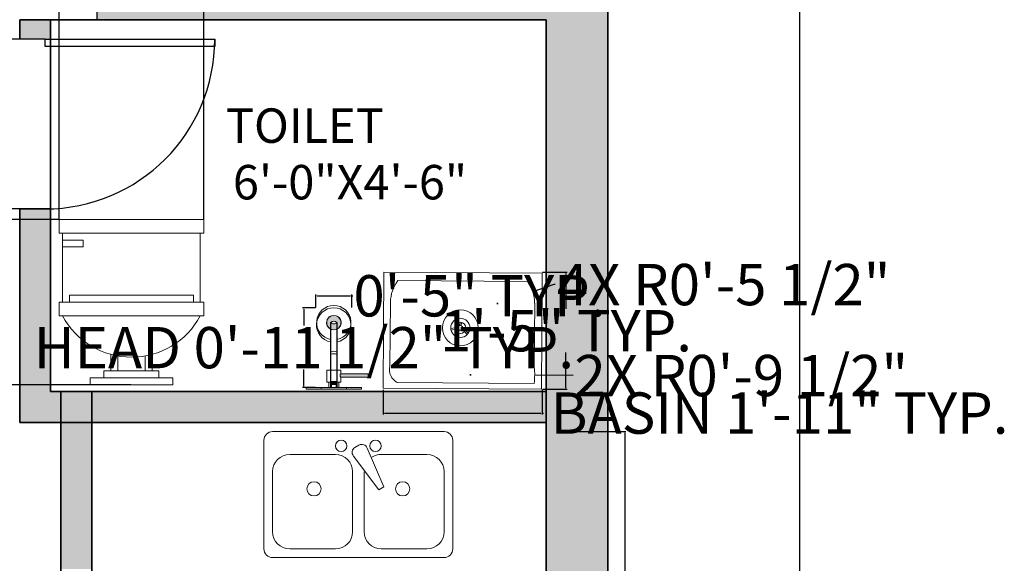
# Model space of a CAD drawing. Units: inches. Extents: x 143233372 to 143233714, y 112671713 to 112672292.
# Tile 5 of 7: x 143233571 to 143233714, y 112672013 to 112672092. Entities that reach past the tile are written whole.
import ezdxf

# ---------------------------------------------------------------- set-up
doc = ezdxf.new("R2010")
doc.units = ezdxf.units.IN
doc.header["$MEASUREMENT"] = 0
doc.layers.get('0').update_dxf_attribs({"color": 104})
for name, color, linetype, lineweight in [('A-ANNO-DIMS', 2, 'Continuous', 18), ('A-AREA-IDEN', 7, 'Continuous', 18), ('doors', 32, 'Continuous', 25), ('PLUMBING FIXTURES', 8, 'Continuous', 18), ('walls', 7, 'Continuous', 35)]:
    doc.layers.add(name, color=color, linetype=linetype, lineweight=lineweight)
doc.layers.add('A-WALL-PATT', color=18, linetype='Continuous', lineweight=9, true_color=0x000000)
doc.styles.add('ATT', font='TXT')
doc.styles.get("Standard").update_dxf_attribs({"font": 'arial.ttf'})
doc.dimstyles.get("Standard").update_dxf_attribs({"dimtxt": 6, "dimasz": 0.18, "dimexe": 0.18, "dimexo": 0.0625, "dimgap": 0.09, "dimtad": 0, "dimtih": 1, "dimtoh": 1, "dimzin": 0, "dimdsep": 46, "dimlunit": 3, "dimtxsty": 'Standard', "dimcen": 0.09, "dimadec": 0, "dimazin": 0, "dimtfac": 1, "dimtofl": 0, "dimtmove": 0, "dimatfit": 3, "dimfxl": 1, "dimtolj": 1, "dimtzin": 0, "dimarcsym": 0})

# ---------------------------------------------------------------- blocks, each defined once
blk = doc.blocks.new('15PSNK10')
at = {"color": 0, "linetype": 'ByBlock'}
for p, q in [((20.5, 16.5), (1.5, 16.5)), ((0, 15), (0, -15)), ((7, 15), (17.5, 15)), ((22, -15), (22, 15)), ((4, 4), (4, 12)), ((20.5, 12), (20.5, 4)), ((2.37, -0.1), (2.77, 0.6)), ((10.18, -3.57), (4.27, 0.87)), ((17.5, 1), (7, 1)), ((2.88, -1.54), (9.68, -4.43)), ((7.04, -1), (17.5, -1)), ((4, -12), (4, -4)), ((9.68, -4.43), (10.18, -3.57)), ((20.5, -4), (20.5, -12)), ((17.5, -15), (7, -15)), ((1.5, -16.5), (20.5, -16.5))]:
    blk.add_line(p, q, dxfattribs=at)
for centre, radius in [((10, 7.75), 1.25), ((2.5, 3), 1), ((2.5, -3), 1), ((10, -7.75), 1.25)]:
    blk.add_circle(centre, radius, dxfattribs=at)
for centre, radius, start, end in [((1.5, 15), 1.5, 90, 180), ((20.5, 15), 1.5, 0, 90), ((7, 12), 3, 90, 180), ((17.5, 12), 3, 0, 90), ((7, 4), 3, 180, 270), ((17.5, 4), 3, 270, 0), ((3.63, 0.1), 1, 50.5377, 150), ((3.23, -0.6), 1, 150, 249.4623), ((17.5, -4), 3, 0, 90), ((7, -4), 3, 146.607, 180), ((7, -12), 3, 180, 270), ((17.5, -12), 3, 270, 0), ((1.5, -15), 1.5, 180, 270), ((20.5, -15), 1.5, 270, 0)]:
    blk.add_arc(centre, radius, start, end, dxfattribs=at)
at = {"color": 0, "linetype": 'ByBlock', "style": 'ATT'}
for tag, p, flags in [('ITEM', (0, -26), 3), ('ROOM_NUMBER', (0, -35), 1)]:
    blk.add_attdef(tag, p, '', height=6, dxfattribs=dict(at, flags=flags))
blk = doc.blocks.new('*U19')
for p, q in [((-10, 22), (-10, 12)), ((10, 12), (10, 22)), ((-10, 21), (-7, 21)), ((-7, 21), (-7, 20)), ((-7, 20), (-10, 20)), ((9, 13), (-9, 13)), ((-9, 13), (-9, 12)), ((9, 12), (9, 13)), ((10.5, 12), (-10.5, 12)), ((-10.5, 10), (-10.5, 12)), ((10.5, 12), (10.5, 10)), ((10.5, 10), (-10.5, 10)), ((-3, 4.4065), (-3, 2)), ((3, 2), (3, 4.4065)), ((-2, 2), (-2, 4.1658)), ((2, 4.1658), (2, 2)), ((4, 2), (-4, 2)), ((-4, 2), (-4, 1)), ((4, 1), (4, 2))]:
    blk.add_line(p, q)
for points in [[(10.5, 22), (10.5, 24), (-10.5, 24), (-10.5, 22)], [(6, 0), (6, 1), (-6, 1), (-6, 0)]]:
    blk.add_lwpolyline(points, close=True)
blk.add_arc((0, 15.3333), 11.3333, 208.0725, 331.9275)
blk = doc.blocks.new('O.H SHOWER-PL')
at = {"layer": 'PLUMBING FIXTURES'}
for points in [[(-1.84, 0), (-1.84, -0.25), (1.84, -0.25), (1.84, 0)], [(0.46, -8.72), (0.46, -9.67, -0.422337), (-0.46, -9.67), (-0.46, -8.72, 4.325472)]]:
    blk.add_hatch(color=256, dxfattribs=at).paths.add_polyline_path(points)
for p, q in [((-1.84, 0), (-1.84, -0.25)), ((1.84, 0), (-1.84, 0)), ((1.84, 0), (1.84, -0.25)), ((1.84, -0.25), (-1.84, -0.25)), ((-0.46, -0.25), (-0.46, -9.67)), ((0.46, -0.25), (0.46, -9.67))]:
    blk.add_line(p, q, dxfattribs=at)
for centre, radius, start, end in [((0, -4.48), 1.03, 243.53, 296.47), ((0, -9.67), 2.5, 100.61, 79.39), ((0, -9.67), 1.05, 116.0349, 63.9652), ((0, -9.22), 0.643, 224.2078, 315.7922)]:
    blk.add_arc(centre, radius, start, end, dxfattribs=at)
blk = doc.blocks.new('DIVERTER-PL')
at = {"layer": 'PLUMBING FIXTURES'}
for points in [[(4, 0), (-4, 0), (-4, -0.25), (4, -0.25)], [(0.38, -1.14), (0.38, -0.7), (-0.37, -0.7), (-0.37, -1.14)], [(1, -1.75, 0.30818), (1, -2.25), (5, -2.25), (5, -1.75)]]:
    blk.add_hatch(color=256, dxfattribs=at).paths.add_polyline_path(points)
for p, q in [((-4, 0), (-4, -0.25)), ((-4, 0), (4, 0)), ((4, 0), (4, -0.25)), ((-4, -0.25), (4, -0.25)), ((-4, -0.25), (4, -0.25)), ((-1, -1.05), (-0.37, -1.05)), ((-1, -1.05), (-1, -2.75)), ((-0.75, -0.25), (-0.75, -1.05)), ((-0.37, -0.7), (0.38, -0.7)), ((-0.37, -0.7), (-0.37, -1.14)), ((-0.37, -1.14), (0.38, -1.14)), ((-0.32, -0.7), (-0.32, -0.25)), ((0.32, -0.7), (0.32, -0.25)), ((0.38, -0.7), (0.38, -1.14)), ((0.38, -1.05), (1, -1.05)), ((0.75, -0.25), (0.75, -1.05)), ((1, -1.05), (1, -1.75)), ((-1, -2.75), (1, -2.75)), ((1, -2.25), (1, -2.75))]:
    blk.add_line(p, q, dxfattribs=at)
at = {"layer": 'PLUMBING FIXTURES', "ltscale": 12}
for p, q in [((1, -1.75), (5, -1.75)), ((1, -2.25), (5, -2.25)), ((5, -2.25), (5, -1.75))]:
    blk.add_line(p, q, dxfattribs=at)
at = {"layer": 'PLUMBING FIXTURES'}
blk.add_arc((1.37, -2), 0.444, 145.7435, 214.2565, dxfattribs=at)
blk = doc.blocks.new('A$C7F153053')
at = {"layer": 'PLUMBING FIXTURES', "xscale": -1, "rotation": 270}
for name in ['DIVERTER-PL', 'O.H SHOWER-PL']:
    blk.add_blockref(name, (12.17, 4), dxfattribs=at)
blk = doc.blocks.new('*U24')
for p, q in [((0, 0), (0, -6)), ((40, 0), (40, -6))]:
    blk.add_line(p, q)
blk.add_lwpolyline([(0, 0), (0, 40), (1.75, 40), (1.75, 0)], close=True)
blk.add_arc((0, 0), 40, 0, 90)
blk = doc.blocks.new('LAVATORY-RECT')
for p, q in [((0, 0.15), (0.11, 17)), ((0.11, 17), (23.11, 16.85)), ((20.97, 15.65), (2.15, 15.77)), ((23.11, 16.85), (23.1, 15.71)), ((23.1, 15.71), (23, 0)), ((0.99, 3.35), (1.05, 12.64)), ((21.96, 3.21), (22.03, 12.5)), ((10.4, 8.91), (9.84, 8.81)), ((10.52, 8.7), (9.87, 8.58)), ((11.22, 9.73), (11.16, 9.24)), ((11.36, 9.22), (11.4, 9.7)), ((11.97, 8.6), (12.36, 8.13)), ((11.84, 8.39), (12.22, 7.95)), ((23, 0), (0, 0.15)), ((21.95, 0.84), (2.06, 0.97))]:
    blk.add_line(p, q)
for radius in [2.61, 1.39, 0.816, 0.338]:
    blk.add_circle((11.22, 8.91), radius)
for centre, radius, start, end in [((6.46, 12.5), 5.4, 142.7525, 178.5493), ((16.62, 12.43), 5.4, 0.6949, 36.4918), ((3, 2.82), 2.08, 165.2338, 242.9258), ((12.7, 2.09), 9.33, 352.3124, 6.9318)]:
    blk.add_arc(centre, radius, start, end)
blk = doc.blocks.new('SHOWER-ARM-AND-HEAD')
blk.add_hatch(color=256).paths.add_polyline_path([(2.05, 10.36), (2.05, 9.42, 0.422337), (2.97, 9.42), (2.97, 10.36, -4.325472)])
blk.add_hatch(color=256).paths.add_polyline_path([(2.05, 10.36), (2.05, 9.42, 0.422337), (2.97, 9.42), (2.97, 10.36, -4.325472)])
blk.add_hatch(color=256).paths.add_polyline_path([(2.05, 10.36), (2.05, 9.42, 0.422337), (2.97, 9.42), (2.97, 10.36, -4.325472)])
blk.add_hatch(color=256).paths.add_polyline_path([(2.05, 10.36), (2.05, 9.42, 0.422337), (2.97, 9.42), (2.97, 10.36, -4.325472)])
blk.add_hatch(color=256).paths.add_polyline_path([(2.05, 10.36), (2.05, 9.42, 0.422337), (2.97, 9.42), (2.97, 10.36, -4.325472)])
blk.add_hatch(color=256).paths.add_polyline_path([(2.05, 10.36), (2.05, 9.42, 0.422337), (2.97, 9.42), (2.97, 10.36, -4.325472)])
blk.add_hatch(color=256).paths.add_polyline_path([(2.05, 10.36), (2.05, 9.42, 0.422337), (2.97, 9.42), (2.97, 10.36, -4.325472)])
blk.add_hatch(color=256).paths.add_polyline_path([(2.05, 10.36), (2.05, 9.42, 0.422337), (2.97, 9.42), (2.97, 10.36, -4.325472)])
blk.add_hatch(color=256).paths.add_polyline_path([(2.05, 10.36), (2.05, 9.42, 0.422337), (2.97, 9.42), (2.97, 10.36, -4.325472)])
blk.add_hatch(color=256).paths.add_polyline_path([(2.05, 10.36), (2.05, 9.42, 0.422337), (2.97, 9.42), (2.97, 10.36, -4.325472)])
blk.add_hatch(color=256).paths.add_polyline_path([(2.05, 10.36), (2.05, 9.42, 0.422337), (2.97, 9.42), (2.97, 10.36, -4.325472)])
blk.add_hatch(color=256).paths.add_polyline_path([(2.05, 10.36), (2.05, 9.42, 0.422337), (2.97, 9.42), (2.97, 10.36, -4.325472)])
blk.add_hatch(color=256).paths.add_polyline_path([(2.05, 10.36), (2.05, 9.42, 0.422337), (2.97, 9.42), (2.97, 10.36, -4.325472)])
blk.add_hatch(color=256).paths.add_polyline_path([(2.05, 10.36), (2.05, 9.42, 0.422337), (2.97, 9.42), (2.97, 10.36, -4.325472)])
blk.add_hatch(color=256).paths.add_polyline_path([(2.05, 10.36), (2.05, 9.42, 0.422337), (2.97, 9.42), (2.97, 10.36, -4.325472)])
blk.add_hatch(color=256).paths.add_polyline_path([(2.05, 10.36), (2.05, 9.42, 0.422337), (2.97, 9.42), (2.97, 10.36, -4.325472)])
blk.add_hatch(color=256).paths.add_polyline_path([(2.05, 10.36), (2.05, 9.42, 0.422337), (2.97, 9.42), (2.97, 10.36, -4.325472)])
blk.add_hatch(color=256).paths.add_polyline_path([(2.05, 10.36), (2.05, 9.42, 0.422337), (2.97, 9.42), (2.97, 10.36, -4.325472)])
blk.add_hatch(color=256).paths.add_polyline_path([(2.05, 10.36), (2.05, 9.42, 0.422337), (2.97, 9.42), (2.97, 10.36, -4.325472)])
blk.add_hatch(color=256).paths.add_polyline_path([(2.05, 10.36), (2.05, 9.42, 0.422337), (2.97, 9.42), (2.97, 10.36, -4.325472)])
blk.add_hatch(color=256).paths.add_polyline_path([(2.05, 10.36), (2.05, 9.42, 0.422337), (2.97, 9.42), (2.97, 10.36, -4.325472)])
blk.add_hatch(color=256).paths.add_polyline_path([(2.05, 10.36), (2.05, 9.42, 0.422337), (2.97, 9.42), (2.97, 10.36, -4.325472)])
blk.add_hatch(color=256).paths.add_polyline_path([(2.05, 10.36), (2.05, 9.42, 0.422337), (2.97, 9.42), (2.97, 10.36, -4.325472)])
blk.add_hatch(color=256).paths.add_polyline_path([(2.05, 10.36), (2.05, 9.42, 0.422337), (2.97, 9.42), (2.97, 10.36, -4.325472)])
blk.add_hatch(color=256).paths.add_polyline_path([(2.05, 10.36), (2.05, 9.42, 0.422337), (2.97, 9.42), (2.97, 10.36, -4.325472)])
blk.add_hatch(color=256).paths.add_polyline_path([(2.05, 10.36), (2.05, 9.42, 0.422337), (2.97, 9.42), (2.97, 10.36, -4.325472)])
blk.add_hatch(color=256).paths.add_polyline_path([(2.05, 10.36), (2.05, 9.42, 0.422337), (2.97, 9.42), (2.97, 10.36, -4.325472)])
blk.add_hatch(color=256).paths.add_polyline_path([(2.05, 10.36), (2.05, 9.42, 0.422337), (2.97, 9.42), (2.97, 10.36, -4.325472)])
blk.add_hatch(color=256).paths.add_polyline_path([(2.05, 10.36), (2.05, 9.42, 0.422337), (2.97, 9.42), (2.97, 10.36, -4.325472)])
blk.add_hatch(color=256).paths.add_polyline_path([(2.05, 10.36), (2.05, 9.42, 0.422337), (2.97, 9.42), (2.97, 10.36, -4.325472)])
blk.add_hatch(color=256).paths.add_polyline_path([(2.05, 10.36), (2.05, 9.42, 0.422337), (2.97, 9.42), (2.97, 10.36, -4.325472)])
blk.add_hatch(color=256).paths.add_polyline_path([(2.05, 10.36), (2.05, 9.42, 0.422337), (2.97, 9.42), (2.97, 10.36, -4.325472)])
blk.add_hatch(color=256).paths.add_polyline_path([(2.05, 10.36), (2.05, 9.42, 0.422337), (2.97, 9.42), (2.97, 10.36, -4.325472)])
blk.add_hatch(color=256).paths.add_polyline_path([(2.05, 10.36), (2.05, 9.42, 0.422337), (2.97, 9.42), (2.97, 10.36, -4.325472)])
blk.add_hatch(color=256).paths.add_polyline_path([(2.05, 10.36), (2.05, 9.42, 0.422337), (2.97, 9.42), (2.97, 10.36, -4.325472)])
blk.add_hatch(color=256).paths.add_polyline_path([(2.05, 10.36), (2.05, 9.42, 0.422337), (2.97, 9.42), (2.97, 10.36, -4.325472)])
blk.add_hatch(color=256).paths.add_polyline_path([(2.05, 10.36), (2.05, 9.42, 0.422337), (2.97, 9.42), (2.97, 10.36, -4.325472)])
blk.add_hatch(color=256).paths.add_polyline_path([(2.05, 10.36), (2.05, 9.42, 0.422337), (2.97, 9.42), (2.97, 10.36, -4.325472)])
for p, q in [((2.05, 0), (2.05, 9.42)), ((2.05, 0), (2.05, 9.42)), ((2.05, 0), (2.05, 9.42)), ((2.05, 0), (2.05, 9.42)), ((2.05, 0), (2.05, 9.42)), ((2.05, 0), (2.05, 9.42)), ((2.05, 0), (2.05, 9.42)), ((2.05, 0), (2.05, 9.42)), ((2.05, 0), (2.05, 9.42)), ((2.05, 0), (2.05, 9.42)), ((2.05, 0), (2.05, 9.42)), ((2.05, 0), (2.05, 9.42)), ((2.05, 0), (2.05, 9.42)), ((2.05, 0), (2.05, 9.42)), ((2.05, 0), (2.05, 9.42)), ((2.05, 0), (2.05, 9.42)), ((2.05, 0), (2.05, 9.42)), ((2.05, 0), (2.05, 9.42)), ((2.05, 0), (2.05, 9.42)), ((2.05, 0), (2.05, 9.42)), ((2.05, 0), (2.05, 9.42)), ((2.05, 0), (2.05, 9.42)), ((2.05, 0), (2.05, 9.42)), ((2.05, 0), (2.05, 9.42)), ((2.05, 0), (2.05, 9.42)), ((2.05, 0), (2.05, 9.42)), ((2.05, 0), (2.05, 9.42)), ((2.05, 0), (2.05, 9.42)), ((2.05, 0), (2.05, 9.42)), ((2.05, 0), (2.05, 9.42)), ((2.05, 0), (2.05, 9.42)), ((2.05, 0), (2.05, 9.42)), ((2.05, 0), (2.05, 9.42)), ((2.05, 0), (2.05, 9.42)), ((2.05, 0), (2.05, 9.42)), ((2.05, 0), (2.05, 9.42)), ((2.05, 0), (2.05, 9.42)), ((2.05, 0), (2.05, 9.42)), ((2.97, 0), (2.97, 9.42)), ((2.97, 0), (2.97, 9.42)), ((2.97, 0), (2.97, 9.42)), ((2.97, 0), (2.97, 9.42)), ((2.97, 0), (2.97, 9.42)), ((2.97, 0), (2.97, 9.42)), ((2.97, 0), (2.97, 9.42)), ((2.97, 0), (2.97, 9.42)), ((2.97, 0), (2.97, 9.42)), ((2.97, 0), (2.97, 9.42)), ((2.97, 0), (2.97, 9.42)), ((2.97, 0), (2.97, 9.42)), ((2.97, 0), (2.97, 9.42)), ((2.97, 0), (2.97, 9.42)), ((2.97, 0), (2.97, 9.42)), ((2.97, 0), (2.97, 9.42)), ((2.97, 0), (2.97, 9.42)), ((2.97, 0), (2.97, 9.42)), ((2.97, 0), (2.97, 9.42)), ((2.97, 0), (2.97, 9.42)), ((2.97, 0), (2.97, 9.42)), ((2.97, 0), (2.97, 9.42)), ((2.97, 0), (2.97, 9.42)), ((2.97, 0), (2.97, 9.42)), ((2.97, 0), (2.97, 9.42)), ((2.97, 0), (2.97, 9.42)), ((2.97, 0), (2.97, 9.42)), ((2.97, 0), (2.97, 9.42)), ((2.97, 0), (2.97, 9.42)), ((2.97, 0), (2.97, 9.42)), ((2.97, 0), (2.97, 9.42)), ((2.97, 0), (2.97, 9.42)), ((2.97, 0), (2.97, 9.42)), ((2.97, 0), (2.97, 9.42)), ((2.97, 0), (2.97, 9.42)), ((2.97, 0), (2.97, 9.42)), ((2.97, 0), (2.97, 9.42)), ((2.97, 0), (2.97, 9.42))]:
    blk.add_line(p, q)
for centre, radius, start, end in [((2.5, 9.07), 2.5, 280.61, 259.39), ((2.5, 9.07), 2.5, 280.61, 259.39), ((2.5, 9.07), 2.5, 280.61, 259.39), ((2.5, 9.07), 2.5, 280.61, 259.39), ((2.5, 9.07), 2.5, 280.61, 259.39), ((2.5, 9.07), 2.5, 280.61, 259.39), ((2.5, 9.07), 2.5, 280.61, 259.39), ((2.5, 9.07), 2.5, 280.61, 259.39), ((2.5, 9.07), 2.5, 280.61, 259.39), ((2.5, 9.07), 2.5, 280.61, 259.39), ((2.5, 9.07), 2.5, 280.61, 259.39), ((2.5, 9.07), 2.5, 280.61, 259.39), ((2.5, 9.07), 2.5, 280.61, 259.39), ((2.5, 9.07), 2.5, 280.61, 259.39), ((2.5, 9.07), 2.5, 280.61, 259.39), ((2.5, 9.07), 2.5, 280.61, 259.39), ((2.5, 9.07), 2.5, 280.61, 259.39), ((2.5, 9.07), 2.5, 280.61, 259.39), ((2.5, 9.07), 2.5, 280.61, 259.39), ((2.5, 9.07), 2.5, 280.61, 259.39), ((2.5, 9.07), 2.5, 280.61, 259.39), ((2.5, 9.07), 2.5, 280.61, 259.39), ((2.5, 9.07), 2.5, 280.61, 259.39), ((2.5, 9.07), 2.5, 280.61, 259.39), ((2.5, 9.07), 2.5, 280.61, 259.39), ((2.5, 9.07), 2.5, 280.61, 259.39), ((2.5, 9.07), 2.5, 280.61, 259.39), ((2.5, 9.07), 2.5, 280.61, 259.39), ((2.5, 9.07), 2.5, 280.61, 259.39), ((2.5, 9.07), 2.5, 280.61, 259.39), ((2.5, 9.07), 2.5, 280.61, 259.39), ((2.5, 9.07), 2.5, 280.61, 259.39), ((2.5, 9.07), 2.5, 280.61, 259.39), ((2.5, 9.07), 2.5, 280.61, 259.39), ((2.5, 9.07), 2.5, 280.61, 259.39), ((2.5, 9.07), 2.5, 280.61, 259.39), ((2.5, 9.07), 2.5, 280.61, 259.39), ((2.5, 9.07), 2.5, 280.61, 259.39), ((2.51, 9.42), 1.05, 116.0348, 63.9651), ((2.51, 9.42), 1.05, 116.0348, 63.9651), ((2.51, 9.42), 1.05, 116.0348, 63.9651), ((2.51, 9.42), 1.05, 116.0348, 63.9651), ((2.51, 9.42), 1.05, 116.0348, 63.9651), ((2.51, 9.42), 1.05, 116.0348, 63.9651), ((2.51, 9.42), 1.05, 116.0348, 63.9651), ((2.51, 9.42), 1.05, 116.0348, 63.9651), ((2.51, 9.42), 1.05, 116.0348, 63.9651), ((2.51, 9.42), 1.05, 116.0348, 63.9651), ((2.51, 9.42), 1.05, 116.0348, 63.9651), ((2.51, 9.42), 1.05, 116.0348, 63.9651), ((2.51, 9.42), 1.05, 116.0348, 63.9651), ((2.51, 9.42), 1.05, 116.0348, 63.9651), ((2.51, 9.42), 1.05, 116.0348, 63.9651), ((2.51, 9.42), 1.05, 116.0348, 63.9651), ((2.51, 9.42), 1.05, 116.0348, 63.9651), ((2.51, 9.42), 1.05, 116.0348, 63.9651), ((2.51, 9.42), 1.05, 116.0348, 63.9651), ((2.51, 9.42), 1.05, 116.0348, 63.9651), ((2.51, 9.42), 1.05, 116.0348, 63.9651), ((2.51, 9.42), 1.05, 116.0348, 63.9651), ((2.51, 9.42), 1.05, 116.0348, 63.9651), ((2.51, 9.42), 1.05, 116.0348, 63.9651), ((2.51, 9.42), 1.05, 116.0348, 63.9651), ((2.51, 9.42), 1.05, 116.0348, 63.9651), ((2.51, 9.42), 1.05, 116.0348, 63.9651), ((2.51, 9.42), 1.05, 116.0348, 63.9651), ((2.51, 9.42), 1.05, 116.0348, 63.9651), ((2.51, 9.42), 1.05, 116.0348, 63.9651), ((2.51, 9.42), 1.05, 116.0348, 63.9651), ((2.51, 9.42), 1.05, 116.0348, 63.9651), ((2.51, 9.42), 1.05, 116.0348, 63.9651), ((2.51, 9.42), 1.05, 116.0348, 63.9651), ((2.51, 9.42), 1.05, 116.0348, 63.9651), ((2.51, 9.42), 1.05, 116.0348, 63.9651), ((2.51, 9.42), 1.05, 116.0348, 63.9651), ((2.51, 9.42), 1.05, 116.0348, 63.9651), ((2.51, 9.87), 0.643, 224.2078, 315.7922), ((2.51, 9.87), 0.643, 224.2078, 315.7922), ((2.51, 9.87), 0.643, 224.2078, 315.7922), ((2.51, 9.87), 0.643, 224.2078, 315.7922), ((2.51, 9.87), 0.643, 224.2078, 315.7922), ((2.51, 9.87), 0.643, 224.2078, 315.7922), ((2.51, 9.87), 0.643, 224.2078, 315.7922), ((2.51, 9.87), 0.643, 224.2078, 315.7922), ((2.51, 9.87), 0.643, 224.2078, 315.7922), ((2.51, 9.87), 0.643, 224.2078, 315.7922), ((2.51, 9.87), 0.643, 224.2078, 315.7922), ((2.51, 9.87), 0.643, 224.2078, 315.7922), ((2.51, 9.87), 0.643, 224.2078, 315.7922), ((2.51, 9.87), 0.643, 224.2078, 315.7922), ((2.51, 9.87), 0.643, 224.2078, 315.7922), ((2.51, 9.87), 0.643, 224.2078, 315.7922), ((2.51, 9.87), 0.643, 224.2078, 315.7922), ((2.51, 9.87), 0.643, 224.2078, 315.7922), ((2.51, 9.87), 0.643, 224.2078, 315.7922), ((2.51, 9.87), 0.643, 224.2078, 315.7922), ((2.51, 9.87), 0.643, 224.2078, 315.7922), ((2.51, 9.87), 0.643, 224.2078, 315.7922), ((2.51, 9.87), 0.643, 224.2078, 315.7922), ((2.51, 9.87), 0.643, 224.2078, 315.7922), ((2.51, 9.87), 0.643, 224.2078, 315.7922), ((2.51, 9.87), 0.643, 224.2078, 315.7922), ((2.51, 9.87), 0.643, 224.2078, 315.7922), ((2.51, 9.87), 0.643, 224.2078, 315.7922), ((2.51, 9.87), 0.643, 224.2078, 315.7922), ((2.51, 9.87), 0.643, 224.2078, 315.7922), ((2.51, 9.87), 0.643, 224.2078, 315.7922), ((2.51, 9.87), 0.643, 224.2078, 315.7922), ((2.51, 9.87), 0.643, 224.2078, 315.7922), ((2.51, 9.87), 0.643, 224.2078, 315.7922), ((2.51, 9.87), 0.643, 224.2078, 315.7922), ((2.51, 9.87), 0.643, 224.2078, 315.7922), ((2.51, 9.87), 0.643, 224.2078, 315.7922), ((2.51, 9.87), 0.643, 224.2078, 315.7922), ((2.5, 3.88), 1.03, 63.53, 116.47), ((2.5, 3.88), 1.03, 63.53, 116.47), ((2.5, 3.88), 1.03, 63.53, 116.47), ((2.5, 3.88), 1.03, 63.53, 116.47), ((2.5, 3.88), 1.03, 63.53, 116.47), ((2.5, 3.88), 1.03, 63.53, 116.47), ((2.5, 3.88), 1.03, 63.53, 116.47), ((2.5, 3.88), 1.03, 63.53, 116.47), ((2.5, 3.88), 1.03, 63.53, 116.47), ((2.5, 3.88), 1.03, 63.53, 116.47), ((2.5, 3.88), 1.03, 63.53, 116.47), ((2.5, 3.88), 1.03, 63.53, 116.47), ((2.5, 3.88), 1.03, 63.53, 116.47), ((2.5, 3.88), 1.03, 63.53, 116.47), ((2.5, 3.88), 1.03, 63.53, 116.47), ((2.5, 3.88), 1.03, 63.53, 116.47), ((2.5, 3.88), 1.03, 63.53, 116.47), ((2.5, 3.88), 1.03, 63.53, 116.47), ((2.5, 3.88), 1.03, 63.53, 116.47), ((2.5, 3.88), 1.03, 63.53, 116.47), ((2.5, 3.88), 1.03, 63.53, 116.47), ((2.5, 3.88), 1.03, 63.53, 116.47), ((2.5, 3.88), 1.03, 63.53, 116.47), ((2.5, 3.88), 1.03, 63.53, 116.47), ((2.5, 3.88), 1.03, 63.53, 116.47), ((2.5, 3.88), 1.03, 63.53, 116.47), ((2.5, 3.88), 1.03, 63.53, 116.47), ((2.5, 3.88), 1.03, 63.53, 116.47), ((2.5, 3.88), 1.03, 63.53, 116.47), ((2.5, 3.88), 1.03, 63.53, 116.47), ((2.5, 3.88), 1.03, 63.53, 116.47), ((2.5, 3.88), 1.03, 63.53, 116.47), ((2.5, 3.88), 1.03, 63.53, 116.47), ((2.5, 3.88), 1.03, 63.53, 116.47), ((2.5, 3.88), 1.03, 63.53, 116.47), ((2.5, 3.88), 1.03, 63.53, 116.47), ((2.5, 3.88), 1.03, 63.53, 116.47), ((2.5, 3.88), 1.03, 63.53, 116.47)]:
    blk.add_arc(centre, radius, start, end)
blk = doc.blocks.new('*D51')
at = {"layer": 'A-ANNO-DIMS', "color": 0, "lineweight": -2, "transparency": 16777216}
for p, q in [((143233623.6, 112672037.96), (143233623.6, 112672034.38)), ((143233646.71, 112672037.96), (143233646.71, 112672034.38)), ((143233623.78, 112672034.56), (143233646.53, 112672034.56)), ((143233646.71, 112672034.56), (143233646.89, 112672034.56))]:
    blk.add_line(p, q, dxfattribs=at)
at = {"layer": 'A-ANNO-DIMS', "color": 0, "transparency": 16777216}
for points in [[(143233623.78, 112672034.59), (143233623.78, 112672034.53), (143233623.6, 112672034.56)], [(143233646.53, 112672034.59), (143233646.53, 112672034.53), (143233646.71, 112672034.56)]]:
    blk.add_solid(points, dxfattribs=at)
at = {"layer": 'Defpoints', "color": 0, "transparency": 16777216}
for p in [(143233623.6, 112672038.02), (143233646.71, 112672038.02), (143233646.71, 112672034.56)]:
    blk.add_point(p, dxfattribs=at)
at = {"layer": 'A-ANNO-DIMS', "color": 0, "transparency": 16777216, "insert": (143233681.21, 112672034.56), "char_height": 6, "attachment_point": 5}
blk.add_mtext('\\A1;BASIN 1\'-11" TYP.', dxfattribs=at)
blk = doc.blocks.new('*D52')
at = {"layer": 'A-ANNO-DIMS', "color": 0, "lineweight": -2, "transparency": 16777216}
for p, q in [((143233646.77, 112672055.02), (143233650.36, 112672055.02)), ((143233650.18, 112672054.84), (143233650.18, 112672049.68)), ((143233650.18, 112672038.2), (143233650.18, 112672043.37)), ((143233646.77, 112672038.02), (143233650.36, 112672038.02))]:
    blk.add_line(p, q, dxfattribs=at)
at = {"layer": 'A-ANNO-DIMS', "color": 0, "transparency": 16777216}
for points in [[(143233650.15, 112672054.84), (143233650.21, 112672054.84), (143233650.18, 112672055.02)], [(143233650.15, 112672038.2), (143233650.21, 112672038.2), (143233650.18, 112672038.02)]]:
    blk.add_solid(points, dxfattribs=at)
at = {"layer": 'Defpoints', "color": 0, "transparency": 16777216}
for p in [(143233646.71, 112672055.02), (143233650.18, 112672055.02), (143233646.71, 112672038.02)]:
    blk.add_point(p, dxfattribs=at)
at = {"layer": 'A-ANNO-DIMS', "color": 0, "transparency": 16777216, "insert": (143233650.18, 112672046.52), "char_height": 6, "attachment_point": 5}
blk.add_mtext('\\A1;1\'-5" TYP.', dxfattribs=at)
blk = doc.blocks.new('*D53')
at = {"layer": 'A-ANNO-DIMS', "color": 0, "lineweight": -2, "transparency": 16777216}
for p, q in [((143233613.76, 112672049.85), (143233611.91, 112672049.85)), ((143233612.09, 112672049.67), (143233612.09, 112672047.26)), ((143233612.09, 112672038.46), (143233612.09, 112672040.87)), ((143233613.76, 112672038.28), (143233611.91, 112672038.28))]:
    blk.add_line(p, q, dxfattribs=at)
at = {"layer": 'A-ANNO-DIMS', "color": 0, "transparency": 16777216}
for points in [[(143233612.06, 112672049.67), (143233612.12, 112672049.67), (143233612.09, 112672049.85)], [(143233612.06, 112672038.46), (143233612.12, 112672038.46), (143233612.09, 112672038.28)]]:
    blk.add_solid(points, dxfattribs=at)
at = {"layer": 'Defpoints', "color": 0, "transparency": 16777216}
for p in [(143233612.09, 112672049.85), (143233613.82, 112672049.85), (143233613.82, 112672038.28)]:
    blk.add_point(p, dxfattribs=at)
at = {"layer": 'A-ANNO-DIMS', "color": 0, "transparency": 16777216, "insert": (143233612.09, 112672044.06), "char_height": 6, "attachment_point": 5}
blk.add_mtext('\\A1;HEAD 0\'-11 1/2" TYP.', dxfattribs=at)
blk = doc.blocks.new('*D54')
at = {"layer": 'A-ANNO-DIMS', "color": 0, "lineweight": -2, "transparency": 16777216}
for p, q in [((143233613.82, 112672049.91), (143233613.82, 112672051.77)), ((143233614, 112672051.59), (143233618.86, 112672051.59)), ((143233619.04, 112672049.91), (143233619.04, 112672051.77)), ((143233619.04, 112672051.59), (143233619.22, 112672051.59))]:
    blk.add_line(p, q, dxfattribs=at)
at = {"layer": 'A-ANNO-DIMS', "color": 0, "transparency": 16777216}
for points in [[(143233614, 112672051.62), (143233614, 112672051.56), (143233613.82, 112672051.59)], [(143233618.86, 112672051.62), (143233618.86, 112672051.56), (143233619.04, 112672051.59)]]:
    blk.add_solid(points, dxfattribs=at)
at = {"layer": 'Defpoints', "color": 0, "transparency": 16777216}
for p in [(143233619.04, 112672051.59), (143233613.82, 112672049.85), (143233619.04, 112672049.85)]:
    blk.add_point(p, dxfattribs=at)
at = {"layer": 'A-ANNO-DIMS', "color": 0, "transparency": 16777216, "insert": (143233637.6, 112672051.59), "char_height": 6, "attachment_point": 5}
blk.add_mtext('\\A1;0\'-5" TYP.', dxfattribs=at)
blk = doc.blocks.new('*D57')
at = {"layer": 'A-ANNO-DIMS', "color": 0, "lineweight": -2, "transparency": 16777216}
for p, q in [((143233650.58, 112672031.88), (143233658.89, 112672031.88)), ((143233658.71, 112672031.7), (143233658.71, 112672007.75)), ((143233658.71, 112671977.41), (143233658.71, 112672001.36)), ((143233650.58, 112671977.23), (143233658.89, 112671977.23))]:
    blk.add_line(p, q, dxfattribs=at)
at = {"layer": 'A-ANNO-DIMS', "color": 0, "transparency": 16777216}
for points in [[(143233658.68, 112672031.7), (143233658.74, 112672031.7), (143233658.71, 112672031.88)], [(143233658.68, 112671977.41), (143233658.74, 112671977.41), (143233658.71, 112671977.23)]]:
    blk.add_solid(points, dxfattribs=at)
at = {"layer": 'Defpoints', "color": 0, "transparency": 16777216}
for p in [(143233650.52, 112672031.88), (143233650.52, 112671977.23), (143233658.71, 112671977.23)]:
    blk.add_point(p, dxfattribs=at)
at = {"layer": 'A-ANNO-DIMS', "color": 0, "transparency": 16777216, "insert": (143233658.71, 112672004.55), "char_height": 6, "attachment_point": 5}
blk.add_mtext('\\A1;SINK UNIT 4\'-6 1/2"', dxfattribs=at)
blk = doc.blocks.new('*D63')
at = {"layer": 'A-ANNO-DIMS', "color": 0, "lineweight": -2, "transparency": 16777216}
for p, q in [((143233656.35, 112672249.18), (143233684.29, 112672249.18)), ((143233684.11, 112672249), (143233684.11, 112671999.82)), ((143233684.11, 112671744.43), (143233684.11, 112671993.61)), ((143233656.35, 112671744.25), (143233684.29, 112671744.25))]:
    blk.add_line(p, q, dxfattribs=at)
at = {"layer": 'A-ANNO-DIMS', "color": 0, "transparency": 16777216}
for points in [[(143233684.08, 112672249), (143233684.14, 112672249), (143233684.11, 112672249.18)], [(143233684.08, 112671744.43), (143233684.14, 112671744.43), (143233684.11, 112671744.25)]]:
    blk.add_solid(points, dxfattribs=at)
at = {"layer": 'Defpoints', "color": 0, "transparency": 16777216}
for p in [(143233656.28, 112672249.18), (143233656.28, 112671744.25), (143233684.11, 112671744.25)]:
    blk.add_point(p, dxfattribs=at)
at = {"layer": 'A-ANNO-DIMS', "color": 0, "transparency": 16777216, "insert": (143233684.11, 112671996.72), "char_height": 6, "attachment_point": 5}
blk.add_mtext('\\A1;42\'-1"', dxfattribs=at)
blk = doc.blocks.new('*D70')
at = {"layer": 'A-ANNO-DIMS', "color": 0, "lineweight": -2, "transparency": 16777216}
for p, q in [((143233574.42, 112672088.85), (143233389.09, 112672088.85)), ((143233389.27, 112672088.67), (143233389.27, 112672079.72)), ((143233389.27, 112672064.38), (143233389.27, 112672073.33)), ((143233575.22, 112672064.2), (143233389.09, 112672064.2))]:
    blk.add_line(p, q, dxfattribs=at)
at = {"layer": 'A-ANNO-DIMS', "color": 0, "transparency": 16777216}
for points in [[(143233389.24, 112672088.67), (143233389.3, 112672088.67), (143233389.27, 112672088.85)], [(143233389.24, 112672064.38), (143233389.3, 112672064.38), (143233389.27, 112672064.2)]]:
    blk.add_solid(points, dxfattribs=at)
at = {"layer": 'Defpoints', "color": 0, "transparency": 16777216}
for p in [(143233574.48, 112672088.85), (143233389.27, 112672064.2), (143233575.28, 112672064.2)]:
    blk.add_point(p, dxfattribs=at)
at = {"layer": 'A-ANNO-DIMS', "color": 0, "transparency": 16777216, "insert": (143233389.27, 112672076.53), "char_height": 6, "attachment_point": 5}
blk.add_mtext('\\A1;2\'-0 1/2"', dxfattribs=at)
blk = doc.blocks.new('*D71')
at = {"layer": 'A-ANNO-DIMS', "color": 0, "lineweight": -2, "transparency": 16777216}
for p, q in [((143233576.53, 112672062.74), (143233576.53, 112672283.7)), ((143233576.71, 112672283.52), (143233579.24, 112672283.52)), ((143233597.35, 112672283.52), (143233594.81, 112672283.52)), ((143233597.53, 112672062.74), (143233597.53, 112672283.7))]:
    blk.add_line(p, q, dxfattribs=at)
at = {"layer": 'A-ANNO-DIMS', "color": 0, "transparency": 16777216}
for points in [[(143233576.71, 112672283.55), (143233576.71, 112672283.49), (143233576.53, 112672283.52)], [(143233597.35, 112672283.55), (143233597.35, 112672283.49), (143233597.53, 112672283.52)]]:
    blk.add_solid(points, dxfattribs=at)
at = {"layer": 'Defpoints', "color": 0, "transparency": 16777216}
for p in [(143233597.53, 112672283.52), (143233576.53, 112672062.68), (143233597.53, 112672062.68)]:
    blk.add_point(p, dxfattribs=at)
at = {"layer": 'A-ANNO-DIMS', "color": 0, "transparency": 16777216, "insert": (143233587.03, 112672283.52), "char_height": 6, "attachment_point": 5}
blk.add_mtext('\\A1;1\'-9"', dxfattribs=at)
blk = doc.blocks.new('*D72')
at = {"layer": 'A-ANNO-DIMS', "color": 0, "lineweight": -2, "transparency": 16777216}
for p, q in [((143233576.46, 112672062.68), (143233389.09, 112672062.68)), ((143233389.27, 112672062.5), (143233389.27, 112672053.84)), ((143233389.27, 112672038.86), (143233389.27, 112672047.53)), ((143233586.96, 112672038.68), (143233389.09, 112672038.68))]:
    blk.add_line(p, q, dxfattribs=at)
at = {"layer": 'A-ANNO-DIMS', "color": 0, "transparency": 16777216}
for points in [[(143233389.24, 112672062.5), (143233389.3, 112672062.5), (143233389.27, 112672062.68)], [(143233389.24, 112672038.86), (143233389.3, 112672038.86), (143233389.27, 112672038.68)]]:
    blk.add_solid(points, dxfattribs=at)
at = {"layer": 'Defpoints', "color": 0, "transparency": 16777216}
for p in [(143233576.53, 112672062.68), (143233389.27, 112672038.68), (143233587.03, 112672038.68)]:
    blk.add_point(p, dxfattribs=at)
at = {"layer": 'A-ANNO-DIMS', "color": 0, "transparency": 16777216, "insert": (143233389.27, 112672050.68), "char_height": 6, "attachment_point": 5}
blk.add_mtext('\\A1;2\'-0"', dxfattribs=at)
blk = doc.blocks.new('*D75')
at = {"layer": 'A-ANNO-DIMS', "color": 0, "lineweight": -2, "transparency": 16777216}
for p, q in [((143233636.22, 112672040.11), (143233636.4, 112672040.11)), ((143233636.31, 112672040.02), (143233636.31, 112672040.2)), ((143233651.23, 112672040.01), (143233645.82, 112672040.05))]:
    blk.add_line(p, q, dxfattribs=at)
at = {"layer": 'A-ANNO-DIMS', "color": 0, "transparency": 16777216}
blk.add_solid([(143233645.82, 112672040.08), (143233645.82, 112672040.02), (143233645.64, 112672040.05)], dxfattribs=at)
at = {"layer": 'Defpoints', "color": 0, "transparency": 16777216}
for p in [(143233636.31, 112672040.11), (143233645.64, 112672040.05)]:
    blk.add_point(p, dxfattribs=at)
at = {"layer": 'A-ANNO-DIMS', "color": 0, "transparency": 16777216, "insert": (143233675.66, 112672040.01), "char_height": 6, "attachment_point": 5}
blk.add_mtext('\\A1;2X R0\'-9 1/2"', dxfattribs=at)
blk = doc.blocks.new('*D76')
at = {"layer": 'A-ANNO-DIMS', "color": 0, "lineweight": -2, "transparency": 16777216}
for p, q in [((143233648.42, 112672053.22), (143233645.52, 112672052.24)), ((143233648.6, 112672053.22), (143233648.42, 112672053.22)), ((143233640.14, 112672050.46), (143233640.32, 112672050.46)), ((143233640.23, 112672050.37), (143233640.23, 112672050.55))]:
    blk.add_line(p, q, dxfattribs=at)
at = {"layer": 'A-ANNO-DIMS', "color": 0, "transparency": 16777216}
blk.add_solid([(143233645.51, 112672052.27), (143233645.53, 112672052.21), (143233645.35, 112672052.18)], dxfattribs=at)
at = {"layer": 'Defpoints', "color": 0, "transparency": 16777216}
for p in [(143233645.35, 112672052.18), (143233640.23, 112672050.46)]:
    blk.add_point(p, dxfattribs=at)
at = {"layer": 'A-ANNO-DIMS', "color": 0, "transparency": 16777216, "insert": (143233673.09, 112672053.22), "char_height": 6, "attachment_point": 5}
blk.add_mtext('\\A1;4X R0\'-5 1/2"', dxfattribs=at)

msp = doc.modelspace()

# ---------------------------------------------------------------- hatches: boundary and pattern name
at = {"layer": 'A-WALL-PATT'}
h = msp.add_hatch(color=256, dxfattribs=at)
h.dxf.hatch_style = 1
h.paths.add_polyline_path([(143233656.285, 112672249.182), (143233647.285, 112672249.182), (143233647.285, 112672240.182), (143233656.285, 112672240.182)])
h.paths.add_polyline_path([(143233647.285, 112672249.182), (143233618.333, 112672249.182), (143233618.333, 112672240.182), (143233647.285, 112672240.182)])
h.paths.add_polyline_path([(143233656.285, 112672240.182), (143233647.285, 112672240.182), (143233647.285, 112672096.182), (143233656.285, 112672096.182)])
h.paths.add_polyline_path([(143233656.285, 112672096.182), (143233647.285, 112672096.182), (143233647.285, 112672091.682), (143233656.285, 112672091.682)])
h.paths.add_polyline_path([(143233647.285, 112672096.182), (143233581.998, 112672096.182), (143233581.998, 112672091.682), (143233647.285, 112672091.682)])
h.paths.add_polyline_path([(143233656.285, 112672091.682), (143233647.285, 112672091.682), (143233647.285, 112672037.682), (143233656.285, 112672037.682)])
h.paths.add_polyline_path([(143233656.285, 112672037.682), (143233647.285, 112672037.682), (143233647.285, 112672033.182), (143233656.285, 112672033.182)])
h.paths.add_polyline_path([(143233656.285, 112672033.182), (143233647.285, 112672033.182), (143233647.285, 112672006.032), (143233656.285, 112672006.032)])
h = msp.add_hatch(color=256, dxfattribs=at)
h.dxf.hatch_style = 1
h.paths.add_polyline_path([(143233575.285, 112672091.682), (143233570.785, 112672091.682), (143233570.785, 112672088.851), (143233574.482, 112672088.851), (143233575.285, 112672088.851)])
h = msp.add_hatch(color=256, dxfattribs=at)
h.dxf.hatch_style = 1
h.paths.add_polyline_path([(143233581.285, 112672037.682), (143233576.785, 112672037.682), (143233576.785, 112672033.182), (143233581.285, 112672033.182)])
h.paths.add_polyline_path([(143233647.285, 112672037.682), (143233581.285, 112672037.682), (143233581.285, 112672033.182), (143233581.285, 112672033.182), (143233647.285, 112672033.182)])
h.paths.add_polyline_path([(143233575.285, 112672064.202), (143233570.785, 112672064.202), (143233570.785, 112672033.182), (143233576.785, 112672033.182), (143233576.785, 112672037.682), (143233575.285, 112672037.682)])
h = msp.add_hatch(color=256, dxfattribs=at)
h.dxf.hatch_style = 1
h.paths.add_polyline_path([(143233549.785, 112671901.182), (143233541.241, 112671901.182), (143233541.241, 112671897.787), (143233541.241, 112671896.682), (143233545.285, 112671896.682), (143233545.285, 112671848.682), (143233549.785, 112671848.682)])
h.paths.add_polyline_path([(143233581.285, 112672033.182), (143233576.785, 112672033.182), (143233576.785, 112672011.912), (143233581.285, 112672011.912)])

# ---------------------------------------------------------------- linework, layer by layer
at = {"layer": 'walls'}
for p, q in [((143233656.285, 112672249.182), (143233656.285, 112671889.182)), ((143233570.785, 112672091.682), (143233570.785, 112672088.851)), ((143233570.785, 112672091.682), (143233647.285, 112672091.682)), ((143233575.285, 112672091.682), (143233575.285, 112672037.682)), ((143233647.285, 112672091.682), (143233647.285, 112672037.682)), ((143233570.785, 112672064.202), (143233570.785, 112672033.182)), ((143233570.785, 112672064.202), (143233575.285, 112672064.202)), ((143233575.285, 112672037.682), (143233647.285, 112672037.682)), ((143233576.785, 112671937.182), (143233576.785, 112672037.682)), ((143233581.285, 112672037.682), (143233581.285, 112671937.182)), ((143233647.285, 112672037.682), (143233647.285, 112671937.182)), ((143233570.785, 112672033.182), (143233647.285, 112672033.182)), ((143233576.785, 112671937.182), (143233576.785, 112672033.182)), ((143233576.785, 112672033.182), (143233581.285, 112672033.182)), ((143233581.285, 112671937.182), (143233581.285, 112672033.182))]:
    msp.add_line(p, q, dxfattribs=at)

# ---------------------------------------------------------------- block references
at = {"layer": 'doors', "xscale": 0.7380496403518878, "yscale": 0.7380496403518878, "zscale": 0.7380496403518878}
msp.add_blockref('*U24', (143233552.476, 112672096.111), dxfattribs=at)
at = {"layer": 'doors', "xscale": 0.6162162669326948, "yscale": 0.6162162669326948, "zscale": 0.6162162669326948, "rotation": 270}
msp.add_blockref('*U24', (143233574.482, 112672088.851), dxfattribs=at)
at = {"layer": 'PLUMBING FIXTURES'}
for name, p in [('*U19', (143233587.026, 112672038.682)), ('LAVATORY-RECT', (143233623.603, 112672038.024))]:
    msp.add_blockref(name, p, dxfattribs=at)
at = {"layer": 'PLUMBING FIXTURES', "ltscale": 35, "rotation": 270}
msp.add_blockref('A$C7F153053', (143233612.439, 112672050.195), dxfattribs=at)
at = {"layer": 'PLUMBING FIXTURES', "rotation": 2.5613209388e-06}
msp.add_blockref('SHOWER-ARM-AND-HEAD', (143233613.932, 112672038.279), dxfattribs=at)
at = {"layer": 'PLUMBING FIXTURES', "xscale": -0.8312046371252371, "yscale": 0.8312046371252371, "zscale": 0.8312046371252371, "rotation": 90}
msp.add_blockref('15PSNK10', (143233620.003, 112672031.875), dxfattribs=at)

# ---------------------------------------------------------------- texts
at = {"layer": 'A-AREA-IDEN'}
for s, p in [('TOILET', (143233600.753, 112672073.803)), ('6\'-0"X4\'-6"', (143233601.771, 112672065.589))]:
    msp.add_text(s, height=5, dxfattribs=at).set_placement(p)

# ---------------------------------------------------------------- dimensions: what is measured, and where the dimension line sits
at = {"layer": 'A-ANNO-DIMS'}
dim = msp.add_linear_dim(base=(143233597.526, 112672283.523), p1=(143233576.526, 112672062.682), p2=(143233597.526, 112672062.682), dimstyle='Standard', override={"dimdec": 1, "dimlfac": 1, "dimrnd": 0, "dimzin": 1, "dimdsep": 46, "dimlunit": 4, "dimfrac": 2}, dxfattribs=at)
dim.commit()
dim.dimension.update_dxf_attribs({"geometry": '*D71', "text_midpoint": (143233587.026, 112672283.523)})
for base, p1, p2, picture, middle in [((143233684.111, 112671744.249), (143233656.285, 112672249.182), (143233656.285, 112671744.249), '*D63', (143233684.111, 112671996.716)), ((143233389.272, 112672064.202), (143233574.482, 112672088.851), (143233575.285, 112672064.202), '*D70', (143233389.272, 112672076.526)), ((143233389.272, 112672038.682), (143233576.526, 112672062.682), (143233587.026, 112672038.682), '*D72', (143233389.272, 112672050.682))]:
    dim = msp.add_linear_dim(base=base, p1=p1, p2=p2, angle=90, dimstyle='Standard', override={"dimdec": 1, "dimlfac": 1, "dimrnd": 0, "dimzin": 1, "dimdsep": 46, "dimlunit": 4, "dimfrac": 2}, dxfattribs=at)
    dim.commit()
    dim.dimension.update_dxf_attribs({"geometry": picture, "text_midpoint": middle})
for center, mpoint, text, picture, middle in [((143233640.226, 112672050.459), (143233645.347, 112672052.182), '4X <>', '*D76', (143233673.094, 112672053.216)), ((143233636.306, 112672040.112), (143233645.636, 112672040.05), '2X <>', '*D75', (143233651.234, 112672040.013))]:
    dim = msp.add_radius_dim(center=center, mpoint=mpoint, text=text, dimstyle='Standard', override={"dimdec": 1, "dimlfac": 1, "dimrnd": 0, "dimzin": 1, "dimdsep": 46, "dimlunit": 4, "dimfrac": 2}, dxfattribs=at)
    dim.commit()
    dim.dimension.update_dxf_attribs({"geometry": picture, "text_midpoint": middle, "dimtype": 164})
for base, p1, p2, angle, text, picture, middle in [((143233612.088, 112672049.85), (143233613.823, 112672038.279), (143233613.823, 112672049.85), 90, 'HEAD <> TYP.', '*D53', (143233612.088, 112672044.065)), ((143233619.044, 112672051.586), (143233613.823, 112672049.85), (143233619.044, 112672049.85), 0, '<> TYP.', '*D54', (143233637.6, 112672051.586)), ((143233650.176, 112672055.023), (143233646.71, 112672038.024), (143233646.71, 112672055.023), 90, '<> TYP.', '*D52', (143233650.176, 112672046.524)), ((143233658.714, 112671977.233), (143233650.518, 112672031.875), (143233650.518, 112671977.233), 270, 'SINK UNIT <>', '*D57', (143233658.714, 112672004.554))]:
    dim = msp.add_linear_dim(base=base, p1=p1, p2=p2, angle=angle, text=text, dimstyle='Standard', override={"dimdec": 1, "dimlfac": 1, "dimrnd": 0, "dimzin": 1, "dimdsep": 46, "dimlunit": 4, "dimfrac": 2}, dxfattribs=at)
    dim.commit()
    dim.dimension.update_dxf_attribs({"geometry": picture, "text_midpoint": middle})
dim = msp.add_linear_dim(base=(143233646.71, 112672034.558), p1=(143233623.603, 112672038.024), p2=(143233646.71, 112672038.024), text='BASIN <> TYP.', dimstyle='Standard', override={"dimdec": 1, "dimlfac": 1, "dimrnd": 0, "dimzin": 1, "dimdsep": 46, "dimlunit": 4, "dimfrac": 2}, dxfattribs=at)
dim.commit()
dim.dimension.update_dxf_attribs({"geometry": '*D51', "text_midpoint": (143233681.205, 112672034.558)})

doc.saveas('drawing.dxf')
